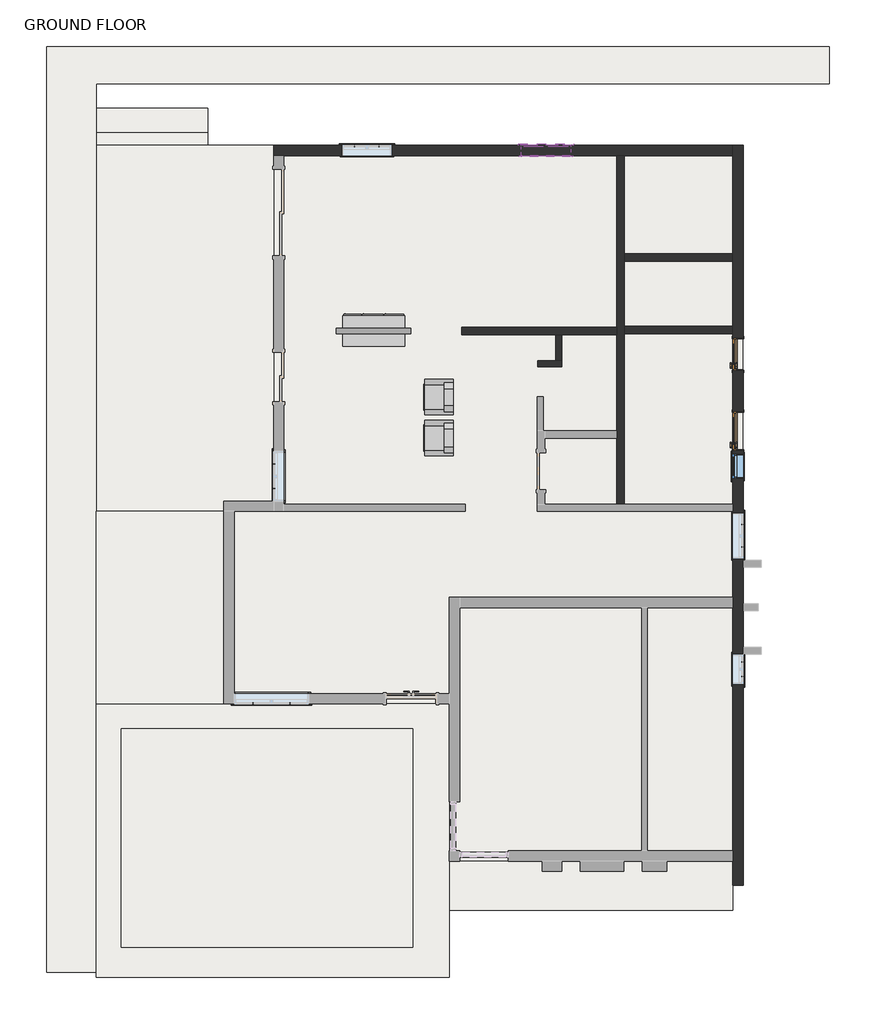
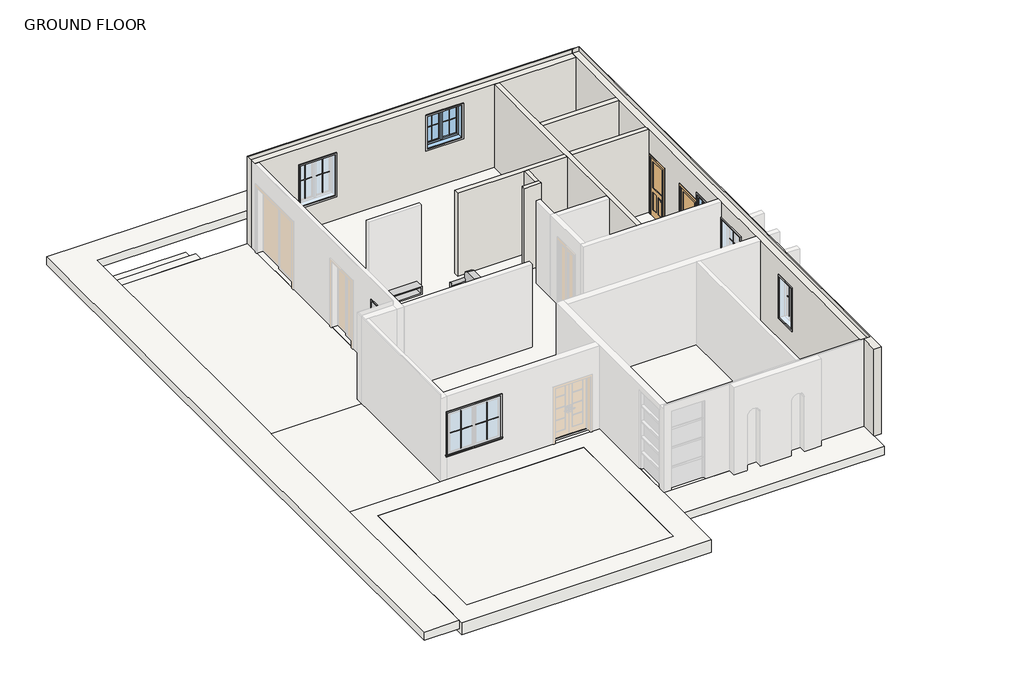
# One storey, part 2 of 2: 27 proxies, 9 slabs, 8 walls, 4 furniture elements, 2 doors, 2 windows.
"""IFC4 building model written with IfcOpenShell, lengths in millimetres."""

from ifc_helpers import new_model, si_unit, frame, origin, origin_with_axes, place, context, project, spatial, polyline, outline, extrude, faceted_brep, transform, mapped, element, save
from components import muntin_pattern_2x2_muntin_pattern_2x2_12159eb8, muntin_pattern_2x2_muntin_pattern_2x2_7b8f790b, muntin_pattern_2x2_muntin_pattern_2x2_a2bda2b8, muntin_pattern_2x2_muntin_pattern_2x2_5c299dc3, muntin_pattern_2x2_muntin_pattern_2x2_e751b040, muntin_pattern_2x2_muntin_pattern_2x2_9cc8fee8, muntin_pattern_2x2_muntin_pattern_2x2_4dfeb3f3, muntin_pattern_2x2_muntin_pattern_2x2_e852a7e4, muntin_pattern_2x2_muntin_pattern_2x2_8031e6f6, muntin_pattern_2x2_muntin_pattern_2x2_6dad3731, muntin_pattern_2x2_muntin_pattern_2x2_a30a3345, trim_window_exterior_flat_with_sill_dc35da0b, trim_window_exterior_flat_with_sill_683e4a0f, trim_window_exterior_flat_with_sill_c22f0c79, trim_window_exterior_flat_with_sill_7cfdd449, trim_window_exterior_flat_with_sill_4912eb0d, trim_window_exterior_flat_with_sill_92b9b949, trim_window_interior_flat_picture_frame_d06e6fc7, trim_window_interior_flat_picture_frame_4c1e0c81, trim_window_interior_flat_picture_frame_d1f4d6ef, trim_window_interior_flat_picture_frame_f1e0b15b, trim_window_interior_flat_picture_frame_978fd00d, trim_window_interior_flat_picture_frame_3bb882cf, door_2_5_90776985, door_3_192038f1, furniture_78335deb, chair_lounge_11461_couch_0866092f, family1_family1_08dda250, window_awning_single_2_9725ec62, window_casement_double_4_window_2_5590f608

model = new_model("IFC4")

# Units and contexts
model_context = context("Model", 3, world=origin())
ifc_project = project(units=[si_unit("LENGTHUNIT", "METRE", prefix="MILLI")], contexts=[model_context])

# Site, building, storey
site = spatial("IfcSite", under=ifc_project)
building = spatial("IfcBuilding", under=site)
storey = spatial("IfcBuildingStorey", under=building, Name="GROUND FLOOR", Elevation=457.2)

# Proxies
placement = place(None, origin())
muntin_pattern_2x2_muntin_pattern_2x2_shape = muntin_pattern_2x2_muntin_pattern_2x2_12159eb8(model_context)
element("IfcBuildingElementProxy", 1, Name="Muntin Pattern_2x2 : Muntin Pattern_2x2", ObjectType="Muntin Pattern_2x2 : Muntin Pattern_2x2", at=placement, inside=storey, context=model_context, shape_type="MappedRepresentation", body=[
    mapped(muntin_pattern_2x2_muntin_pattern_2x2_shape, transform((6234.5834916, 167.7933623, 1441.45), x_axis=(0.0, -1.0, 0.0), y_axis=(1.0, 0.0, 0.0), z_axis=(0.0, 0.0, 1.0))),
])
muntin_pattern_2x2_muntin_pattern_2x2_2_shape = muntin_pattern_2x2_muntin_pattern_2x2_7b8f790b(model_context)
element("IfcBuildingElementProxy", 2, Name="Muntin Pattern_2x2 : Muntin Pattern_2x2", ObjectType="Muntin Pattern_2x2 : Muntin Pattern_2x2", at=placement, inside=storey, context=model_context, shape_type="MappedRepresentation", body=[
    mapped(muntin_pattern_2x2_muntin_pattern_2x2_2_shape, transform((6234.5834916, -387.8316377, 1441.45), x_axis=(0.0, 1.0, 0.0), y_axis=(-1.0, 0.0, 0.0), z_axis=(0.0, 0.0, 1.0))),
])
muntin_pattern_2x2_muntin_pattern_2x2_3_shape = muntin_pattern_2x2_muntin_pattern_2x2_a2bda2b8(model_context)
element("IfcBuildingElementProxy", 3, Name="Muntin Pattern_2x2 : Muntin Pattern_2x2", ObjectType="Muntin Pattern_2x2 : Muntin Pattern_2x2", at=placement, inside=storey, context=model_context, shape_type="MappedRepresentation", body=[
    mapped(muntin_pattern_2x2_muntin_pattern_2x2_3_shape, transform((6234.5834916, -3204.4733398, 1441.45), x_axis=(0.0, -1.0, 0.0), y_axis=(1.0, 0.0, 0.0), z_axis=(0.0, 0.0, 1.0))),
])
muntin_pattern_2x2_muntin_pattern_2x2_4_shape = muntin_pattern_2x2_muntin_pattern_2x2_5c299dc3(model_context)
element("IfcBuildingElementProxy", 4, Name="Muntin Pattern_2x2 : Muntin Pattern_2x2", ObjectType="Muntin Pattern_2x2 : Muntin Pattern_2x2", at=placement, inside=storey, context=model_context, shape_type="MappedRepresentation", body=[
    mapped(muntin_pattern_2x2_muntin_pattern_2x2_4_shape, transform((6234.5834916, -3569.5983398, 1441.45), x_axis=(0.0, 1.0, 0.0), y_axis=(-1.0, 0.0, 0.0), z_axis=(0.0, 0.0, 1.0))),
])
muntin_pattern_2x2_muntin_pattern_2x2_5_shape = muntin_pattern_2x2_muntin_pattern_2x2_e751b040(model_context)
element("IfcBuildingElementProxy", 5, Name="Muntin Pattern_2x2 : Muntin Pattern_2x2", ObjectType="Muntin Pattern_2x2 : Muntin Pattern_2x2", at=placement, inside=storey, context=model_context, shape_type="MappedRepresentation", body=[
    mapped(muntin_pattern_2x2_muntin_pattern_2x2_5_shape, transform((-4883.0879467, -4227.6016767, 1441.45), x_axis=(-1.0, 0.0, 0.0), y_axis=(0.0, -1.0, 0.0), z_axis=(0.0, 0.0, 1.0))),
])
muntin_pattern_2x2_muntin_pattern_2x2_6_shape = muntin_pattern_2x2_muntin_pattern_2x2_9cc8fee8(model_context)
element("IfcBuildingElementProxy", 6, Name="Muntin Pattern_2x2 : Muntin Pattern_2x2", ObjectType="Muntin Pattern_2x2 : Muntin Pattern_2x2", at=placement, inside=storey, context=model_context, shape_type="MappedRepresentation", body=[
    mapped(muntin_pattern_2x2_muntin_pattern_2x2_6_shape, transform((-5794.3129467, -4227.6016767, 1441.45), x_axis=(1.0, 0.0, 0.0), y_axis=(0.0, 1.0, 0.0), z_axis=(0.0, 0.0, 1.0))),
])
muntin_pattern_2x2_muntin_pattern_2x2_7_shape = muntin_pattern_2x2_muntin_pattern_2x2_4dfeb3f3(model_context)
element("IfcBuildingElementProxy", 7, Name="Muntin Pattern_2x2 : Muntin Pattern_2x2", ObjectType="Muntin Pattern_2x2 : Muntin Pattern_2x2", at=placement, inside=storey, context=model_context, shape_type="MappedRepresentation", body=[
    mapped(muntin_pattern_2x2_muntin_pattern_2x2_7_shape, transform((1101.9313637, 9469.4685985, 2027.05), x_axis=(1.0, 0.0, 0.0), y_axis=(0.0, 1.0, 0.0), z_axis=(0.0, 0.0, 1.0))),
])
muntin_pattern_2x2_muntin_pattern_2x2_8_shape = muntin_pattern_2x2_muntin_pattern_2x2_e852a7e4(model_context)
element("IfcBuildingElementProxy", 8, Name="Muntin Pattern_2x2 : Muntin Pattern_2x2", ObjectType="Muntin Pattern_2x2 : Muntin Pattern_2x2", at=placement, inside=storey, context=model_context, shape_type="MappedRepresentation", body=[
    mapped(muntin_pattern_2x2_muntin_pattern_2x2_8_shape, transform((1708.3563637, 9469.4685985, 2027.05), x_axis=(-1.0, 0.0, 0.0), y_axis=(0.0, -1.0, 0.0), z_axis=(0.0, 0.0, 1.0))),
])
muntin_pattern_2x2_muntin_pattern_2x2_9_shape = muntin_pattern_2x2_muntin_pattern_2x2_8031e6f6(model_context)
element("IfcBuildingElementProxy", 9, Name="Muntin Pattern_2x2 : Muntin Pattern_2x2", ObjectType="Muntin Pattern_2x2 : Muntin Pattern_2x2", at=placement, inside=storey, context=model_context, shape_type="MappedRepresentation", body=[
    mapped(muntin_pattern_2x2_muntin_pattern_2x2_9_shape, transform((5999.6334916, 1597.0935985, 1441.45), x_axis=(0.0, 1.0, 0.0), y_axis=(-1.0, 0.0, 0.0), z_axis=(0.0, 0.0, 1.0))),
])
muntin_pattern_2x2_muntin_pattern_2x2_10_shape = muntin_pattern_2x2_muntin_pattern_2x2_6dad3731(model_context)
element("IfcBuildingElementProxy", 10, Name="Muntin Pattern_2x2 : Muntin Pattern_2x2", ObjectType="Muntin Pattern_2x2 : Muntin Pattern_2x2", at=placement, inside=storey, context=model_context, shape_type="MappedRepresentation", body=[
    mapped(muntin_pattern_2x2_muntin_pattern_2x2_10_shape, transform((-5278.2311363, 1047.5096373, 1441.45), x_axis=(0.0, 1.0, 0.0), y_axis=(-1.0, 0.0, 0.0), z_axis=(0.0, 0.0, 1.0))),
])
element("IfcBuildingElementProxy", 11, Name="Muntin Pattern_2x2 : Muntin Pattern_2x2", ObjectType="Muntin Pattern_2x2 : Muntin Pattern_2x2", at=placement, inside=storey, context=model_context, shape_type="MappedRepresentation", body=[
    mapped(muntin_pattern_2x2_muntin_pattern_2x2_10_shape, transform((-3299.7482334, 9469.4685985, 1441.45), x_axis=(1.0, 0.0, 0.0), y_axis=(0.0, 1.0, 0.0), z_axis=(0.0, 0.0, 1.0))),
])
muntin_pattern_2x2_muntin_pattern_2x2_11_shape = muntin_pattern_2x2_muntin_pattern_2x2_a30a3345(model_context)
element("IfcBuildingElementProxy", 12, Name="Muntin Pattern_2x2 : Muntin Pattern_2x2", ObjectType="Muntin Pattern_2x2 : Muntin Pattern_2x2", at=placement, inside=storey, context=model_context, shape_type="MappedRepresentation", body=[
    mapped(muntin_pattern_2x2_muntin_pattern_2x2_11_shape, transform((-5278.2311363, 1653.9346373, 1441.45), x_axis=(0.0, -1.0, 0.0), y_axis=(1.0, 0.0, 0.0), z_axis=(0.0, 0.0, 1.0))),
])
element("IfcBuildingElementProxy", 13, Name="Muntin Pattern_2x2 : Muntin Pattern_2x2", ObjectType="Muntin Pattern_2x2 : Muntin Pattern_2x2", at=placement, inside=storey, context=model_context, shape_type="MappedRepresentation", body=[
    mapped(muntin_pattern_2x2_muntin_pattern_2x2_11_shape, transform((-2693.3232334, 9469.4685985, 1441.45), x_axis=(-1.0, 0.0, 0.0), y_axis=(0.0, -1.0, 0.0), z_axis=(0.0, 0.0, 1.0))),
])
trim_window_exterior_flat_with_sill_shape = trim_window_exterior_flat_with_sill_dc35da0b(model_context)
element("IfcBuildingElementProxy", 14, Name="Trim-Window-Exterior-Flat : with Sill", ObjectType="Trim-Window-Exterior-Flat : with Sill", at=placement, inside=storey, context=model_context, shape_type="MappedRepresentation", body=[
    mapped(trim_window_exterior_flat_with_sill_shape, transform((6244.1084916, -110.0191377, 2895.6), x_axis=(0.0, 1.0, 0.0), y_axis=(0.0, 0.0, 1.0), z_axis=(1.0, 0.0, 0.0))),
])
trim_window_exterior_flat_with_sill_2_shape = trim_window_exterior_flat_with_sill_683e4a0f(model_context)
element("IfcBuildingElementProxy", 15, Name="Trim-Window-Exterior-Flat : with Sill", ObjectType="Trim-Window-Exterior-Flat : with Sill", at=placement, inside=storey, context=model_context, shape_type="MappedRepresentation", body=[
    mapped(trim_window_exterior_flat_with_sill_2_shape, transform((6244.1084916, -3387.0358398, 2895.6), x_axis=(0.0, 1.0, 0.0), y_axis=(0.0, 0.0, 1.0), z_axis=(1.0, 0.0, 0.0))),
])
trim_window_exterior_flat_with_sill_3_shape = trim_window_exterior_flat_with_sill_c22f0c79(model_context)
element("IfcBuildingElementProxy", 16, Name="Trim-Window-Exterior-Flat : with Sill", ObjectType="Trim-Window-Exterior-Flat : with Sill", at=placement, inside=storey, context=model_context, shape_type="MappedRepresentation", body=[
    mapped(trim_window_exterior_flat_with_sill_3_shape, transform((-5338.7004467, -4237.1266767, 2895.6), x_axis=(1.0, 0.0, 0.0), y_axis=(0.0, 0.0, 1.0), z_axis=(0.0, -1.0, 0.0))),
])
trim_window_exterior_flat_with_sill_4_shape = trim_window_exterior_flat_with_sill_7cfdd449(model_context)
element("IfcBuildingElementProxy", 17, Name="Trim-Window-Exterior-Flat : with Sill", ObjectType="Trim-Window-Exterior-Flat : with Sill", at=placement, inside=storey, context=model_context, shape_type="MappedRepresentation", body=[
    mapped(trim_window_exterior_flat_with_sill_4_shape, transform((1405.1438637, 9478.9935985, 3176.4), x_axis=(-1.0, 0.0, 0.0), y_axis=(0.0, 0.0, 1.0), z_axis=(0.0, 1.0, 0.0))),
])
trim_window_exterior_flat_with_sill_5_shape = trim_window_exterior_flat_with_sill_4912eb0d(model_context)
element("IfcBuildingElementProxy", 18, Name="Trim-Window-Exterior-Flat : with Sill", ObjectType="Trim-Window-Exterior-Flat : with Sill", at=placement, inside=storey, context=model_context, shape_type="MappedRepresentation", body=[
    mapped(trim_window_exterior_flat_with_sill_5_shape, transform((5990.1084916, 1597.0935985, 2895.6), x_axis=(0.0, -1.0, 0.0), y_axis=(0.0, 0.0, 1.0), z_axis=(-1.0, 0.0, 0.0))),
])
trim_window_exterior_flat_with_sill_6_shape = trim_window_exterior_flat_with_sill_92b9b949(model_context)
element("IfcBuildingElementProxy", 19, Name="Trim-Window-Exterior-Flat : with Sill", ObjectType="Trim-Window-Exterior-Flat : with Sill", at=placement, inside=storey, context=model_context, shape_type="MappedRepresentation", body=[
    mapped(trim_window_exterior_flat_with_sill_6_shape, transform((-5287.7561363, 1350.7221373, 2895.6), x_axis=(0.0, -1.0, 0.0), y_axis=(0.0, 0.0, 1.0), z_axis=(-1.0, 0.0, 0.0))),
])
element("IfcBuildingElementProxy", 20, Name="Trim-Window-Exterior-Flat : with Sill", ObjectType="Trim-Window-Exterior-Flat : with Sill", at=placement, inside=storey, context=model_context, shape_type="MappedRepresentation", body=[
    mapped(trim_window_exterior_flat_with_sill_6_shape, transform((-2996.5357334, 9478.9935985, 2895.6), x_axis=(-1.0, 0.0, 0.0), y_axis=(0.0, 0.0, 1.0), z_axis=(0.0, 1.0, 0.0))),
])
trim_window_interior_flat_picture_frame_shape = trim_window_interior_flat_picture_frame_d06e6fc7(model_context)
element("IfcBuildingElementProxy", 21, Name="Trim-Window-Interior-Flat : Picture Frame", ObjectType="Trim-Window-Interior-Flat : Picture Frame", at=placement, inside=storey, context=model_context, shape_type="MappedRepresentation", body=[
    mapped(trim_window_interior_flat_picture_frame_shape, transform((5990.1084916, -110.0191377, 2895.6), x_axis=(0.0, -1.0, 0.0), y_axis=(0.0, 0.0, 1.0), z_axis=(-1.0, 0.0, 0.0))),
])
trim_window_interior_flat_picture_frame_2_shape = trim_window_interior_flat_picture_frame_4c1e0c81(model_context)
element("IfcBuildingElementProxy", 22, Name="Trim-Window-Interior-Flat : Picture Frame", ObjectType="Trim-Window-Interior-Flat : Picture Frame", at=placement, inside=storey, context=model_context, shape_type="MappedRepresentation", body=[
    mapped(trim_window_interior_flat_picture_frame_2_shape, transform((5990.1084916, -3387.0358398, 2895.6), x_axis=(0.0, -1.0, 0.0), y_axis=(0.0, 0.0, 1.0), z_axis=(-1.0, 0.0, 0.0))),
])
trim_window_interior_flat_picture_frame_3_shape = trim_window_interior_flat_picture_frame_d1f4d6ef(model_context)
element("IfcBuildingElementProxy", 23, Name="Trim-Window-Interior-Flat : Picture Frame", ObjectType="Trim-Window-Interior-Flat : Picture Frame", at=placement, inside=storey, context=model_context, shape_type="MappedRepresentation", body=[
    mapped(trim_window_interior_flat_picture_frame_3_shape, transform((-5338.7004467, -3983.1266767, 2895.6), x_axis=(-1.0, 0.0, 0.0), y_axis=(0.0, 0.0, 1.0), z_axis=(0.0, 1.0, 0.0))),
])
trim_window_interior_flat_picture_frame_4_shape = trim_window_interior_flat_picture_frame_f1e0b15b(model_context)
element("IfcBuildingElementProxy", 24, Name="Trim-Window-Interior-Flat : Picture Frame", ObjectType="Trim-Window-Interior-Flat : Picture Frame", at=placement, inside=storey, context=model_context, shape_type="MappedRepresentation", body=[
    mapped(trim_window_interior_flat_picture_frame_4_shape, transform((1405.1438637, 9224.9935985, 3176.4), x_axis=(1.0, 0.0, 0.0), y_axis=(0.0, 0.0, 1.0), z_axis=(0.0, -1.0, 0.0))),
])
trim_window_interior_flat_picture_frame_5_shape = trim_window_interior_flat_picture_frame_978fd00d(model_context)
element("IfcBuildingElementProxy", 25, Name="Trim-Window-Interior-Flat : Picture Frame", ObjectType="Trim-Window-Interior-Flat : Picture Frame", at=placement, inside=storey, context=model_context, shape_type="MappedRepresentation", body=[
    mapped(trim_window_interior_flat_picture_frame_5_shape, transform((6244.1084916, 1597.0935985, 2895.6), x_axis=(0.0, 1.0, 0.0), y_axis=(0.0, 0.0, 1.0), z_axis=(1.0, 0.0, 0.0))),
])
trim_window_interior_flat_picture_frame_6_shape = trim_window_interior_flat_picture_frame_3bb882cf(model_context)
element("IfcBuildingElementProxy", 26, Name="Trim-Window-Interior-Flat : Picture Frame", ObjectType="Trim-Window-Interior-Flat : Picture Frame", at=placement, inside=storey, context=model_context, shape_type="MappedRepresentation", body=[
    mapped(trim_window_interior_flat_picture_frame_6_shape, transform((-5033.7561363, 1350.7221373, 2895.6), x_axis=(0.0, 1.0, 0.0), y_axis=(0.0, 0.0, 1.0), z_axis=(1.0, 0.0, 0.0))),
])
element("IfcBuildingElementProxy", 27, Name="Trim-Window-Interior-Flat : Picture Frame", ObjectType="Trim-Window-Interior-Flat : Picture Frame", at=placement, inside=storey, context=model_context, shape_type="MappedRepresentation", body=[
    mapped(trim_window_interior_flat_picture_frame_6_shape, transform((-2996.5357334, 9224.9935985, 2895.6), x_axis=(1.0, 0.0, 0.0), y_axis=(0.0, 0.0, 1.0), z_axis=(0.0, -1.0, 0.0))),
])

# Doors
door_2_5_shape = door_2_5_90776985(model_context)
element("IfcDoor", 28, ObjectType="2.5'", at=placement, inside=storey, context=model_context, shape_type="MappedRepresentation", body=[
    mapped(door_2_5_shape, transform((6113.9334916, 4345.0935985, 457.2), x_axis=(0.0, -1.0, 0.0), y_axis=(1.0, 0.0, 0.0), z_axis=(0.0, 0.0, 1.0))),
])
door_3_shape = door_3_192038f1(model_context)
element("IfcDoor", 29, ObjectType="3'", at=placement, inside=storey, context=model_context, shape_type="MappedRepresentation", body=[
    mapped(door_3_shape, transform((6113.9334916, 2460.6935985, 457.2), x_axis=(0.0, -1.0, 0.0), y_axis=(1.0, 0.0, 0.0), z_axis=(0.0, 0.0, 1.0))),
])

# Furniture
furniture_shape = furniture_78335deb(model_context)
element("IfcFurniture", 30, at=placement, inside=storey, context=model_context, shape_type="MappedRepresentation", body=[
    mapped(furniture_shape, transform((-2829.2809093, 5141.7322749, 457.2), x_axis=(-1.0, 0.0, 0.0), y_axis=(0.0, -1.0, 0.0), z_axis=(0.0, 0.0, 1.0))),
])
chair_lounge_11461_couch_shape = chair_lounge_11461_couch_0866092f(model_context)
element("IfcFurniture", 31, ObjectType="Chair-Lounge_11461 : Couch", at=placement, inside=storey, context=model_context, shape_type="MappedRepresentation", body=[
    mapped(chair_lounge_11461_couch_shape, transform((-874.5061363, 2290.7935985, 457.2), x_axis=(0.0, -1.0, 0.0), y_axis=(1.0, 0.0, 0.0), z_axis=(0.0, 0.0, 1.0))),
])
element("IfcFurniture", 32, ObjectType="Chair-Lounge_11461 : Couch", at=placement, inside=storey, context=model_context, shape_type="MappedRepresentation", body=[
    mapped(chair_lounge_11461_couch_shape, transform((-874.5061363, 3294.0935985, 457.2), x_axis=(0.0, -1.0, 0.0), y_axis=(1.0, 0.0, 0.0), z_axis=(0.0, 0.0, 1.0))),
])
family1_family1_shape = family1_family1_08dda250(model_context)
element("IfcFurniture", 33, ObjectType="Family1 : Family1", at=placement, inside=storey, context=model_context, shape_type="MappedRepresentation", body=[
    mapped(family1_family1_shape, transform((-2829.2809093, 4849.6322749, 457.2), x_axis=(-1.0, 0.0, 0.0), y_axis=(0.0, -1.0, 0.0), z_axis=(0.0, 0.0, 1.0))),
])

# Slabs
element("IfcSlab", 34, ObjectType="6\"", at=placement, inside=storey, context=model_context, shape_type="SweptSolid", body=[
    extrude(outline(polyline([(-5287.7561363, 9478.9935985), (-5287.7561363, 741.1221373), (-6507.1004467, 741.1221373), (-6507.1004467, 487.1221375), (-9643.8561363, 487.1221375), (-9643.8561363, 9478.9935985), (-5287.7561363, 9478.9935985)])), origin_with_axes(), (0.0, 0.0, 1.0), 457.2),
])
element("IfcSlab", 35, ObjectType="6\" 3", at=placement, inside=storey, context=model_context, shape_type="SweptSolid", body=[
    extrude(outline(polyline([(-6900.6561363, 9478.9935985), (-9643.8561363, 9478.9935985), (-9643.8561363, 10393.3935985), (-6900.6561363, 10393.3935985), (-6900.6561363, 9478.9935985)])), origin_with_axes(), (0.0, 0.0, 1.0), 152.4),
])
element("IfcSlab", 36, ObjectType="6\" 3", at=placement, inside=storey, context=model_context, shape_type="SweptSolid", body=[
    extrude(outline(polyline([(-6900.6561363, 9478.9935985), (-9643.8561363, 9478.9935985), (-9643.8561363, 9783.7935985), (-6900.6561363, 9783.7935985), (-6900.6561363, 9478.9935985)])), frame((0.0, 0.0, 304.8), z_axis=(0.0, 0.0, 1.0), x_axis=(1.0, 0.0, 0.0)), (0.0, 0.0, 1.0), 152.4),
])
element("IfcSlab", 37, ObjectType="6\" 4", at=placement, inside=storey, context=model_context, shape_type="SweptSolid", body=[
    extrude(outline(polyline([(-6507.1004467, 487.1221375), (-6507.1004467, -4237.1266767), (-9643.8561363, -4237.1266767), (-9643.8561363, 487.1221375), (-6507.1004467, 487.1221375)])), origin_with_axes(), (0.0, 0.0, 1.0), 457.2),
])
element("IfcSlab", 38, ObjectType="6\" 5", at=placement, inside=storey, context=model_context, shape_type="SweptSolid", body=[
    extrude(outline(polyline([(-1864.8415084, -4846.7266767), (-1864.8415084, -10218.7064015), (-9034.2561363, -10218.7064015), (-9034.2561363, -4846.7266767), (-1864.8415084, -4846.7266767)])), origin_with_axes(), (0.0, 0.0, 1.0), 457.2),
])
element("IfcSlab", 39, ObjectType="6\" 6", at=placement, inside=storey, context=model_context, shape_type="SweptSolid", body=[
    extrude(outline(polyline([(-969.7561363, -4237.1266767), (-969.7561363, -10955.3064015), (-9643.8561363, -10955.3064015), (-9643.8561363, -4237.1266767), (-969.7561363, -4237.1266767)]), holes=[polyline([(-1864.8415084, -4846.7266767), (-9034.2561363, -4846.7266767), (-9034.2561363, -10218.7064015), (-1864.8415084, -10218.7064015), (-1864.8415084, -4846.7266767)])]), origin_with_axes(), (0.0, 0.0, 1.0), 457.2),
])
element("IfcSlab", 40, ObjectType="GRASS", at=placement, inside=storey, context=model_context, shape_type="SweptSolid", body=[
    extrude(outline(polyline([(-10863.0561363, -10828.3064015), (-10863.0561363, 11904.6935985), (-9643.8561363, 11904.6935985), (8352.5731195, 11904.6935985), (8352.5731195, 10990.2935985), (-9643.8561363, 10990.2935985), (-9643.8561363, -10828.3064015), (-10863.0561363, -10828.3064015)])), frame((0.0, 0.0, 152.4), z_axis=(0.0, 0.0, 1.0), x_axis=(1.0, 0.0, 0.0)), (0.0, 0.0, 1.0), 304.8),
])
element("IfcSlab", 41, ObjectType="GRASS", at=placement, inside=storey, context=model_context, shape_type="SweptSolid", body=[
    extrude(outline(polyline([(5990.1084916, -9304.3064015), (-969.7561363, -9304.3064015), (-969.7561363, -8097.8064015), (5990.1084916, -8097.8064015), (5990.1084916, -9304.3064015)])), frame((0.0, 0.0, 152.4), z_axis=(0.0, 0.0, 1.0), x_axis=(1.0, 0.0, 0.0)), (0.0, 0.0, 1.0), 304.8),
])
element("IfcSlab", 42, ObjectType="INTERIOR TILES", at=placement, inside=storey, context=model_context, shape_type="Brep", body=[
    faceted_brep([(-5275.0561363, 9466.0221373, 0.0), (6231.1438637, 9466.0221373, 0.0), (6231.1438637, -8085.3778627, 0.0), (5990.1084916, -8085.3778627, 0.0), (-715.7561363, -8085.3778627, 0.0), (-957.0561363, -8085.3778627, 0.0), (-957.0561363, -4224.5778627, 0.0), (-969.7561363, -4224.5778627, 0.0), (-6253.1004467, -4224.5778627, 0.0), (-6494.2561363, -4224.5778627, 0.0), (-6494.2561363, 487.1221373, 0.0), (-6494.2561363, 728.4221373, 0.0), (-5287.7561363, 728.4221373, 0.0), (-5275.0561363, 728.4221373, 0.0), (-5275.0561363, 9224.9935985, 0.0), (-5275.0561363, 9466.0221373, 457.2), (-5275.0561363, 9224.9935985, 457.2), (-5275.0561363, 728.4221373, 457.2), (-5287.7561363, 728.4221373, 457.2), (-6494.2561363, 728.4221373, 457.2), (-6494.2561363, 487.1221373, 457.2), (-6494.2561363, -4224.5778627, 457.2), (-6253.1004467, -4224.5778627, 457.2), (-969.7561363, -4224.5778627, 457.2), (-957.0561363, -4224.5778627, 457.2), (-957.0561363, -8085.3778627, 457.2), (-715.7561363, -8085.3778627, 457.2), (5990.1084916, -8085.3778627, 457.2), (6231.1438637, -8085.3778627, 457.2), (6231.1438637, 9466.0221373, 457.2)], [[[0, 1, 2, 3, 4, 5, 6, 7, 8, 9, 10, 11, 12, 13, 14]], [[15, 16, 17, 18, 19, 20, 21, 22, 23, 24, 25, 26, 27, 28, 29]], [[1, 0, 15, 29]], [[2, 1, 29, 28]], [[5, 4, 3, 2, 28, 27, 26, 25]], [[6, 5, 25, 24]], [[9, 8, 7, 6, 24, 23, 22, 21]], [[11, 10, 9, 21, 20, 19]], [[13, 12, 11, 19, 18, 17]], [[0, 14, 13, 17, 16, 15]]]),
])

# Walls
element("IfcWall", 43, ObjectType="4.5\"", at=placement, inside=storey, context=model_context, shape_type="Brep", body=[
    faceted_brep([(1201.9438637, 4042.9709514, 457.2), (1786.1438637, 4042.9709514, 457.2), (1786.1438637, 4042.9709514, 3505.2), (1201.9438637, 4042.9709514, 3505.2), (1786.1438637, 4182.6709514, 457.2), (1646.4438637, 4182.6709514, 457.2), (1201.9438637, 4182.6709514, 457.2), (1201.9438637, 4182.6709514, 3505.2), (1786.1438637, 4182.6709514, 3505.2)], [[[0, 1, 2, 3]], [[4, 5, 6, 7, 8]], [[1, 0, 6, 5, 4]], [[6, 0, 3, 7]], [[1, 4, 8, 2]], [[3, 2, 8, 7]]]),
])
element("IfcWall", 44, ObjectType="4.5\"", at=placement, inside=storey, context=model_context, shape_type="SweptSolid", body=[
    extrude(outline(polyline([(1786.1438637, 4830.5822749), (1786.1438637, 4182.6709514), (1646.4438637, 4182.6709514), (1646.4438637, 4830.5822749), (1786.1438637, 4830.5822749)])), frame((0.0, 0.0, 457.2), z_axis=(0.0, 0.0, 1.0), x_axis=(1.0, 0.0, 0.0)), (0.0, 0.0, 1.0), 3048.0),
])
element("IfcWall", 45, ObjectType="6\" WALL", at=placement, inside=storey, context=model_context, shape_type="Brep", body=[
    faceted_brep([(3322.8438637, 665.1935985, 457.2), (3322.8438637, 4856.1935985, 457.2), (3322.8438637, 5033.9935985, 457.2), (3322.8438637, 6634.1935985, 457.2), (3322.8438637, 6811.9935985, 457.2), (3322.8438637, 9224.9935985, 457.2), (3322.8438637, 9224.9935985, 3505.2), (3322.8438637, 665.1935985, 3505.2), (3145.0438637, 9224.9935985, 457.2), (3145.0438637, 5008.3822749, 457.2), (3145.0438637, 4830.5822749, 457.2), (3145.0438637, 2468.5935985, 457.2), (3145.0438637, 2290.7935985, 457.2), (3145.0438637, 665.1935985, 457.2), (3145.0438637, 665.1935985, 3505.2), (3145.0438637, 2290.7935985, 3505.2), (3145.0438637, 2468.5935985, 3505.2), (3145.0438637, 4830.5822749, 3505.2), (3145.0438637, 5008.3822749, 3505.2), (3145.0438637, 9224.9935985, 3505.2)], [[[0, 1, 2, 3, 4, 5, 6, 7]], [[8, 9, 10, 11, 12, 13, 14, 15, 16, 17, 18, 19]], [[5, 4, 3, 2, 1, 0, 13, 12, 11, 10, 9, 8]], [[5, 8, 19, 6]], [[13, 0, 7, 14]], [[7, 6, 19, 18, 17, 16, 15, 14]]]),
])
element("IfcWall", 46, ObjectType="6\" WALL", at=placement, inside=storey, context=model_context, shape_type="SweptSolid", body=[
    extrude(outline(polyline([(5990.1084916, 6634.1935985), (3322.8438637, 6634.1935985), (3322.8438637, 6811.9935985), (5990.1084916, 6811.9935985), (5990.1084916, 6634.1935985)])), frame((0.0, 0.0, 457.2), z_axis=(0.0, 0.0, 1.0), x_axis=(1.0, 0.0, 0.0)), (0.0, 0.0, 1.0), 3048.0),
])
element("IfcWall", 47, ObjectType="6\" WALL", at=placement, inside=storey, context=model_context, shape_type="SweptSolid", body=[
    extrude(outline(polyline([(5990.1084916, 4856.1935985), (3322.8438637, 4856.1935985), (3322.8438637, 5033.9935985), (5990.1084916, 5033.9935985), (5990.1084916, 4856.1935985)])), frame((0.0, 0.0, 457.2), z_axis=(0.0, 0.0, 1.0), x_axis=(1.0, 0.0, 0.0)), (0.0, 0.0, 1.0), 3048.0),
])
element("IfcWall", 48, ObjectType="6\" WALL", at=placement, inside=storey, context=model_context, shape_type="Brep", body=[
    faceted_brep([(3145.0438637, 5008.3822749, 457.2), (-664.9561363, 5008.3822749, 457.2), (-664.9561363, 5008.3822749, 3505.2), (3145.0438637, 5008.3822749, 3505.2), (-664.9561363, 4830.5822749, 457.2), (1646.4438637, 4830.5822749, 457.2), (1786.1438637, 4830.5822749, 457.2), (3145.0438637, 4830.5822749, 457.2), (3145.0438637, 4830.5822749, 3505.2), (1786.1438637, 4830.5822749, 3505.2), (1646.4438637, 4830.5822749, 3505.2), (-664.9561363, 4830.5822749, 3505.2)], [[[0, 1, 2, 3]], [[4, 5, 6, 7, 8, 9, 10, 11]], [[1, 0, 7, 6, 5, 4]], [[1, 4, 11, 2]], [[7, 0, 3, 8]], [[3, 2, 11, 10, 9, 8]]]),
])
element("IfcWall", 49, ObjectType="9\"", at=placement, inside=storey, context=model_context, shape_type="Brep", body=[
    faceted_brep([(5990.1084916, -8694.7064015, 457.2), (5990.1084916, -8694.7064015, 3657.6), (5990.1084916, -8097.8064015, 3657.6), (5990.1084916, -8085.1064015, 3657.6), (5990.1084916, -8085.1064015, 3505.2), (5990.1084916, -1874.8064015, 3505.2), (5990.1084916, -1620.8064015, 3505.2), (5990.1084916, 487.3935985, 3505.2), (5990.1084916, 665.1935985, 3505.2), (5990.1084916, 4856.1935985, 3505.2), (5990.1084916, 5033.9935985, 3505.2), (5990.1084916, 6634.1935985, 3505.2), (5990.1084916, 6811.9935985, 3505.2), (5990.1084916, 9466.2935985, 3505.2), (5990.1084916, 9466.2935985, 3657.6), (5990.1084916, 9478.9935985, 3657.6), (5990.1084916, 9478.9935985, 457.2), (5990.1084916, 9224.9935985, 457.2), (5990.1084916, 6811.9935985, 457.2), (5990.1084916, 6634.1935985, 457.2), (5990.1084916, 5033.9935985, 457.2), (5990.1084916, 4856.1935985, 457.2), (5990.1084916, 4751.4935985, 457.2), (5990.1084916, 4751.4935985, 2616.2), (5990.1084916, 3938.6935985, 2616.2), (5990.1084916, 3938.6935985, 457.2), (5990.1084916, 2943.2935985, 457.2), (5990.1084916, 2943.2935985, 2616.2), (5990.1084916, 1978.0935985, 2616.2), (5990.1084916, 1978.0935985, 457.2), (5990.1084916, 665.1935985, 457.2), (5990.1084916, 487.3935985, 457.2), (5990.1084916, -1620.8064015, 457.2), (5990.1084916, -1874.8064015, 457.2), (5990.1084916, -7843.8064015, 457.2), (5990.1084916, -8097.8064015, 457.2), (5990.1084916, -668.8191377, 2895.6), (5990.1084916, -668.8191377, 1371.6), (5990.1084916, 448.7808623, 1371.6), (5990.1084916, 448.7808623, 2895.6), (5990.1084916, -3755.3358398, 2895.6), (5990.1084916, -3755.3358398, 1371.6), (5990.1084916, -3018.7358398, 1371.6), (5990.1084916, -3018.7358398, 2895.6), (5990.1084916, 1901.8935985, 1371.6), (5990.1084916, 1901.8935985, 2895.6), (5990.1084916, 1292.2935985, 2895.6), (5990.1084916, 1292.2935985, 1371.6), (6244.1084916, -8694.7064015, 3657.6), (6244.1084916, -8694.7064015, 457.2), (6244.1084916, -3018.7358398, 457.2), (6244.1084916, -2840.9358398, 457.2), (6244.1084916, -1952.0318739, 457.2), (6244.1084916, -1774.2318739, 457.2), (6244.1084916, -885.2318739, 457.2), (6244.1084916, -707.4318739, 457.2), (6244.1084916, 1978.0935985, 457.2), (6244.1084916, 1978.0935985, 2616.2), (6244.1084916, 2943.2935985, 2616.2), (6244.1084916, 2943.2935985, 457.2), (6244.1084916, 3938.6935985, 457.2), (6244.1084916, 3938.6935985, 2616.2), (6244.1084916, 4751.4935985, 2616.2), (6244.1084916, 4751.4935985, 457.2), (6244.1084916, 9478.9935985, 457.2), (6244.1084916, 9478.9935985, 3657.6), (6244.1084916, -707.4318739, 3657.6), (6244.1084916, -885.2318739, 3657.6), (6244.1084916, -1774.2318739, 3657.6), (6244.1084916, -1952.0318739, 3657.6), (6244.1084916, -2840.9358398, 3657.6), (6244.1084916, -3018.7358398, 3657.6), (6244.1084916, -668.8191377, 1371.6), (6244.1084916, -668.8191377, 2895.6), (6244.1084916, 448.7808623, 2895.6), (6244.1084916, 448.7808623, 1371.6), (6244.1084916, -3755.3358398, 1371.6), (6244.1084916, -3755.3358398, 2895.6), (6244.1084916, -3018.7358398, 2895.6), (6244.1084916, -3018.7358398, 1371.6), (6244.1084916, 1901.8935985, 2895.6), (6244.1084916, 1901.8935985, 1371.6), (6244.1084916, 1292.2935985, 1371.6), (6244.1084916, 1292.2935985, 2895.6), (6218.7084916, 9466.2935985, 3657.6), (6218.7084916, -8085.1064015, 3657.6), (6218.7084916, -8085.1064015, 3505.2), (6218.7084916, 9466.2935985, 3505.2)], [[[0, 1, 2, 3, 4, 5, 6, 7, 8, 9, 10, 11, 12, 13, 14, 15, 16, 17, 18, 19, 20, 21, 22, 23, 24, 25, 26, 27, 28, 29, 30, 31, 32, 33, 34, 35], [36, 37, 38, 39], [40, 41, 42, 43], [44, 45, 46, 47]], [[48, 49, 50, 51, 52, 53, 54, 55, 56, 57, 58, 59, 60, 61, 62, 63, 64, 65, 66, 67, 68, 69, 70, 71], [72, 73, 74, 75], [76, 77, 78, 79], [80, 81, 82, 83]], [[16, 64, 63, 22, 21, 20, 19, 18, 17]], [[49, 0, 35, 34, 33, 32, 31, 30, 29, 56, 55, 54, 53, 52, 51, 50]], [[25, 60, 59, 26]], [[1, 0, 49, 48]], [[48, 71, 70, 69, 68, 67, 66, 65, 15, 14, 84, 85, 3, 2, 1]], [[16, 15, 65, 64]], [[37, 36, 73, 72]], [[38, 37, 72, 75]], [[39, 38, 75, 74]], [[36, 39, 74, 73]], [[41, 40, 77, 76]], [[42, 41, 76, 79]], [[43, 42, 79, 78]], [[40, 43, 78, 77]], [[24, 61, 60, 25]], [[61, 24, 23, 62]], [[62, 23, 22, 63]], [[28, 57, 56, 29]], [[57, 28, 27, 58]], [[58, 27, 26, 59]], [[81, 80, 45, 44]], [[82, 81, 44, 47]], [[83, 82, 47, 46]], [[80, 83, 46, 45]], [[86, 87, 13, 12, 11, 10, 9, 8, 7, 6, 5, 4]], [[87, 86, 85, 84]], [[85, 86, 4, 3]], [[87, 84, 14, 13]]]),
])
element("IfcWall", 50, ObjectType="9\"", at=placement, inside=storey, context=model_context, shape_type="Brep", body=[
    faceted_brep([(5990.1084916, 9478.9935985, 457.2), (-5287.7561363, 9478.9935985, 457.2), (-5287.7561363, 9478.9935985, 3657.6), (5990.1084916, 9478.9935985, 3657.6), (-2386.9357334, 9478.9935985, 1371.6), (-2386.9357334, 9478.9935985, 2895.6), (-3606.1357334, 9478.9935985, 2895.6), (-3606.1357334, 9478.9935985, 1371.6), (2014.7438637, 9478.9935985, 1957.2), (2014.7438637, 9478.9935985, 3176.4), (795.5438637, 9478.9935985, 3176.4), (795.5438637, 9478.9935985, 1957.2), (-5287.7561363, 9224.9935985, 457.2), (-5033.7561363, 9224.9935985, 457.2), (3145.0438637, 9224.9935985, 457.2), (3322.8438637, 9224.9935985, 457.2), (5990.1084916, 9224.9935985, 457.2), (5990.1084916, 9224.9935985, 3505.2), (3322.8438637, 9224.9935985, 3505.2), (3145.0438637, 9224.9935985, 3505.2), (-5033.7561363, 9224.9935985, 3505.2), (-5275.0561363, 9224.9935985, 3505.2), (-5275.0561363, 9224.9935985, 3657.6), (-5287.7561363, 9224.9935985, 3657.6), (-2386.9357334, 9224.9935985, 2895.6), (-2386.9357334, 9224.9935985, 1371.6), (-3606.1357334, 9224.9935985, 1371.6), (-3606.1357334, 9224.9935985, 2895.6), (2014.7438637, 9224.9935985, 3176.4), (2014.7438637, 9224.9935985, 1957.2), (795.5438637, 9224.9935985, 1957.2), (795.5438637, 9224.9935985, 3176.4), (-5275.0561363, 9466.2935985, 3657.6), (5990.1084916, 9466.2935985, 3657.6), (5990.1084916, 9466.2935985, 3505.2), (-5275.0561363, 9466.2935985, 3505.2)], [[[0, 1, 2, 3], [4, 5, 6, 7], [8, 9, 10, 11]], [[12, 13, 14, 15, 16, 17, 18, 19, 20, 21, 22, 23], [24, 25, 26, 27], [28, 29, 30, 31]], [[1, 0, 16, 15, 14, 13, 12]], [[3, 2, 23, 22, 32, 33]], [[0, 3, 33, 34, 17, 16]], [[2, 1, 12, 23]], [[25, 24, 5, 4]], [[26, 25, 4, 7]], [[27, 26, 7, 6]], [[24, 27, 6, 5]], [[8, 29, 28, 9]], [[29, 8, 11, 30]], [[30, 11, 10, 31]], [[9, 28, 31, 10]], [[34, 35, 21, 20, 19, 18, 17]], [[32, 35, 34, 33]], [[35, 32, 22, 21]]]),
])

# Windows
window_awning_single_2_shape = window_awning_single_2_9725ec62(model_context)
element("IfcWindow", 51, ObjectType="Window-Awning-Single : 2'", at=placement, inside=storey, context=model_context, shape_type="MappedRepresentation", body=[
    mapped(window_awning_single_2_shape, transform((6117.1084916, 1597.0935985, 457.2), x_axis=(0.0, 1.0, 0.0), y_axis=(-1.0, 0.0, 0.0), z_axis=(0.0, 0.0, 1.0))),
])
window_casement_double_4_window_2_shape = window_casement_double_4_window_2_5590f608(model_context)
element("IfcWindow", 52, ObjectType="Window-Casement-Double : 4 window 2", at=placement, inside=storey, context=model_context, shape_type="MappedRepresentation", body=[
    mapped(window_casement_double_4_window_2_shape, transform((1405.1438637, 9351.9935985, 1042.8), x_axis=(1.0, 0.0, 0.0), y_axis=(0.0, 1.0, 0.0), z_axis=(0.0, 0.0, 1.0))),
])

save(model, "model.ifc")

# Revit data of these elements
# Type "Muntin Pattern_2x2 : Muntin Pattern_2x2"
#   Width [instance default] = 4' - 0"
#   Thickness = 0' - 0 1/2"
#   Height [instance default] = 4' - 0"
#   Distance = 0' - 0 3/4"
#   Interior Material [instance default] = none
#   Exterior Material [instance default] = none
#   Default Elevation = 0
# Type "Trim-Window-Exterior-Flat : with Sill"
#   Trim Width = 0' - 2 1/4"
#   Trim Thickness_Picture Frame = 0' - 1 1/4"
#   Trim Thickness_with Sill = 0' - 0 3/4"
#   Sill Thickness = 0' - 1 1/4"
#   Opening Width [instance default] = 2' - 0"
#   Opening Height [instance default] = 3' - 0"
#   Default Elevation = 4' - 0"
#   Sill = yes
#   Picture Frame = no
#   Trim Material [instance default] = none
# Type "Trim-Window-Interior-Flat : Picture Frame"
#   Trim Thickness_Picture Frame = 0' - 1 1/4"
#   Trim Width = 0' - 2 1/4"
#   Trim Thickness_with Sill = 0' - 0 3/4"
#   Sill Thickness = 0' - 1 1/4"
#   Opening Width [instance default] = 2' - 0"
#   Opening Height [instance default] = 3' - 0"
#   Default Elevation = 4' - 0"
#   Sill = no
#   Picture Frame = yes
#   Trim Material [instance default] = none
# Type "2.5'"
#   Type Mark = "11"
#   Assembly Code = "B2030100"
#   Analytic Construction = "French door, wood frame with single glass"
#   Top Rail = 0' - 4 3/4"
#   Threshold Offset [instance default] = 0' - 0 1/2"
#   Thickness = 0' - 1 3/8"
#   Thermal Resistance (R) = 1.0696 (h·ft²·°F)/BTU
#   Swing Angle [instance default] = 90.00°
#   Stiles = 0' - 4 3/4"
#   Rough Width = 2' - 8"
#   Rough Height = 7' - 1"
#   Lock Rail = 0' - 7 1/8"
#   Height = 7' - 0"
#   Width = 2' - 6"
#   Heat Transfer Coefficient (U) = 0.9350 BTU/(h·ft²·°F)
#   Door Offset [instance default] = 0' - 0"
#   Bottom Rail = 0' - 9 1/2"
#   Threshold [instance default] = yes
#   Function = 1
#   Exterior Trim [instance default] = yes
#   Trim Material = Cherry
#   Threshold Material = Cherry
#   Panel Material = Cherry
#   Glazing = Glass
#   Frame Material = Cherry
#   Door Handle Material = Aluminum
#   Visual Light Transmittance = 0
#   Solar Heat Gain Coefficient = 0
#   Wall Closure = (empty or 0)
#   Construction Type = (empty or 0)
# Type "3'"
#   Type Mark = "12"
#   Assembly Code = "B2030100"
#   Analytic Construction = "French door, wood frame with single glass"
#   Top Rail = 0' - 4 3/4"
#   Threshold Offset [instance default] = 0' - 0 1/2"
#   Thickness = 0' - 1 3/8"
#   Thermal Resistance (R) = 1.0696 (h·ft²·°F)/BTU
#   Swing Angle [instance default] = 90.00°
#   Stiles = 0' - 4 3/4"
#   Rough Width = 3' - 2"
#   Rough Height = 7' - 1"
#   Lock Rail = 0' - 7 1/8"
#   Height = 7' - 0"
#   Width = 3' - 0"
#   Heat Transfer Coefficient (U) = 0.9350 BTU/(h·ft²·°F)
#   Door Offset [instance default] = 0' - 0"
#   Bottom Rail = 0' - 9 1/2"
#   Threshold [instance default] = yes
#   Function = 1
#   Exterior Trim [instance default] = yes
#   Trim Material = Cherry
#   Threshold Material = Cherry
#   Panel Material = Cherry
#   Glazing = Glass
#   Frame Material = Cherry
#   Door Handle Material = Aluminum
#   Visual Light Transmittance = 0
#   Solar Heat Gain Coefficient = 0
#   Wall Closure = (empty or 0)
#   Construction Type = (empty or 0)
# Type
#   Default Elevation = 0
# Type "Chair-Lounge_11461 : Couch"
#   Default Elevation = 0
#   Assembly Code = ""
# Type "Family1 : Family1"
#   Default Elevation = 0
# Type "6\""
#   Assembly Code = "B1010"
#   Function = 0
#   Layers, outside or top first: 1' - 6" "WOOD FLOOR" (function 1)
# Type "6\" 3"
#   Assembly Code = "B1010"
#   Function = 0
#   Layers, outside or top first: 0' - 6" "Concrete, Cast-in-Place gray" (function 1)
# Type "6\" 4"
#   Assembly Code = "B1010"
#   Function = 0
#   Layers, outside or top first: 1' - 6" "WALKING AREA TILES(1)" (function 1)
# Type "6\" 5"
#   Assembly Code = "B1010"
#   Function = 0
#   Layers, outside or top first: 1' - 6" "WALKING AREA TILES(1)" (function 1)
# Type "6\" 6"
#   Assembly Code = "B1010"
#   Function = 0
#   Layers, outside or top first: 1' - 6" "WALKING AREA TILES" (function 1)
# Type "GRASS"
#   Assembly Code = "B1010"
#   Function = 0
#   Layers, outside or top first: 1' - 0" "Grass" (function 1)
# Type "INTERIOR TILES"
#   Assembly Code = "B1010"
#   Function = 0
#   Layers, outside or top first: 1' - 6" "INTERIOR TILE" (function 1)
# Type "4.5\""
#   Assembly Code = "B2010"
#   Layers, outside or top first: 0' - 0 1/2" no material (function 4); 0' - 4 1/2" "Acoustic Ceiling Tile 24 x 24" (function 1); 0' - 0 1/2" no material (function 4)
# Type "6\" WALL"
#   Assembly Code = "B2010"
#   Layers, outside or top first: 0' - 0 1/2" no material (function 4); 0' - 6" no material (function 1); 0' - 0 1/2" no material (function 4)
# Type "9\""
#   Assembly Code = "B2010"
#   Layers, outside or top first: 0' - 0 1/2" no material (function 4); 0' - 9" no material (function 1); 0' - 0 1/2" no material (function 4)
# Type "Window-Awning-Single : 2'"
#   Type Mark = "24"
#   Fire Rating = "0.5h"
#   Assembly Code = "B2020100"
#   Analytic Construction = "Double glazing - domestic"
#   Window Inset [instance default] = 0' - 0"
#   Wall Thickness [instance default] = 0' - 6"
#   Visual Light Transmittance = 0.81
#   Thermal Resistance (R) = 1.8146 (h·ft²·°F)/BTU
#   Solar Heat Gain Coefficient = 0.76
#   Rough Width = 2' - 0 1/2"
#   Rough Height = 5' - 0 1/2"
#   Interior Wall Closure [instance default] = 0' - 2 1/4"
#   Height = 5' - 0"
#   Heat Transfer Coefficient (U) = 0.5511 BTU/(h·ft²·°F)
#   Frame Extension [instance default] = 0' - 0 1/4"
#   Exterior Wall Closure [instance default] = 0' - 1 1/4"
#   Extension Jamb [instance default] = 0' - 2 1/4"
#   Default Sill Height = 3' - 0"
#   Width = 2' - 0"
#   Muntin Visibility = yes
#   Interior Trim Visibility [instance default] = yes
#   Exterior Trim Visibility [instance default] = yes
#   Extension Jamb Visibility [instance default] = yes
#   Muntin Pattern = Muntin Pattern_2x2 : Muntin Pattern_2x2
#   Interior Trim Material = Wood - Stained
#   Interior Trim = Trim-Window-Interior-Flat : Picture Frame
#   Interior Frame Material = Wood - Stained
#   Glass Panel Material = Glass
#   Exterior Trim Material = Clad - White
#   Exterior Trim = Trim-Window-Exterior-Flat : with Sill
#   Exterior Frame Material = Clad - White
#   Wall Closure = (empty or 0)
# Type "Window-Casement-Double : 4 window 2"
#   Type Mark = "22"
#   Fire Rating = "0.5h"
#   Assembly Code = "B2020100"
#   Analytic Construction = "Double glazing - domestic"
#   Frame Extension [instance default] = 0' - 0 1/4"
#   Window Inset [instance default] = 0' - 0"
#   Wall Thickness [instance default] = 0' - 6"
#   Interior Wall Closure [instance default] = 0' - 2 1/4"
#   Half Width = 2' - 0"
#   Visual Light Transmittance = 0.81
#   Thermal Resistance (R) = 1.8146 (h·ft²·°F)/BTU
#   Solar Heat Gain Coefficient = 0.76
#   Rough Width = 4' - 0 1/2"
#   Rough Height = 4' - 0 1/2"
#   Height = 4' - 0"
#   Heat Transfer Coefficient (U) = 0.5511 BTU/(h·ft²·°F)
#   Exterior Wall Closure [instance default] = 0' - 1 1/4"
#   Extension Jamb [instance default] = 0' - 2 1/4"
#   Default Sill Height = 3' - 0"
#   Width = 4' - 0"
#   Muntin Visibility = yes
#   Interior Trim Visibility [instance default] = yes
#   Exterior Trim Visibility [instance default] = yes
#   Extension Jamb Visibility [instance default] = yes
#   Interior Trim Material = Wood - Stained
#   Muntin Pattern = Muntin Pattern_2x2 : Muntin Pattern_2x2
#   Interior Trim = Trim-Window-Interior-Flat : Picture Frame
#   Interior Frame Material = Wood - Stained
#   Glass Panel Material = Glass
#   Exterior Trim Material = Clad - White
#   Exterior Trim = Trim-Window-Exterior-Flat : with Sill
#   Exterior Frame Material = Clad - White
#   Wall Closure = (empty or 0)
# Elements 1, 2 (IfcBuildingElementProxy, "Muntin Pattern_2x2 : Muntin Pattern_2x2")
#   Width = 1' - 4 5/8"
#   Height = 4' - 6 1/2"
#   Interior Material = Wood - Stained
#   Exterior Material = Clad - White
#   Phase Created = New Construction
#   Materials on its faces: "Clad - White", "Wood - Stained"
# Elements 3, 4 (IfcBuildingElementProxy, "Muntin Pattern_2x2 : Muntin Pattern_2x2")
#   Width = 0' - 9 1/8"
#   Height = 4' - 6 1/2"
#   Interior Material = Wood - Stained
#   Exterior Material = Clad - White
#   Phase Created = New Construction
#   Materials on its faces: "Clad - White", "Wood - Stained"
# Elements 5, 6 (IfcBuildingElementProxy, "Muntin Pattern_2x2 : Muntin Pattern_2x2")
#   Width = 2' - 6 5/8"
#   Height = 4' - 6 1/2"
#   Interior Material = Wood - Stained
#   Exterior Material = Clad - White
#   Phase Created = New Construction
#   Materials on its faces: "Clad - White", "Wood - Stained"
# Elements 7, 8 (IfcBuildingElementProxy, "Muntin Pattern_2x2 : Muntin Pattern_2x2")
#   Width = 1' - 6 5/8"
#   Height = 3' - 6 1/2"
#   Interior Material = Wood - Stained
#   Exterior Material = Clad - White
#   Phase Created = New Construction
#   Materials on its faces: "Clad - White", "Wood - Stained"
# Element 9 (IfcBuildingElementProxy, "Muntin Pattern_2x2 : Muntin Pattern_2x2")
#   Width = 1' - 6 1/2"
#   Height = 4' - 6 1/2"
#   Interior Material = Wood - Stained
#   Exterior Material = Clad - White
#   Phase Created = New Construction
#   Materials on its faces: "Clad - White", "Wood - Stained"
# Elements 10, 11, 12, 13 (IfcBuildingElementProxy, "Muntin Pattern_2x2 : Muntin Pattern_2x2")
#   Width = 1' - 6 5/8"
#   Height = 4' - 6 1/2"
#   Interior Material = Wood - Stained
#   Exterior Material = Clad - White
#   Phase Created = New Construction
#   Materials on its faces: "Clad - White", "Wood - Stained"
# Element 14 (IfcBuildingElementProxy, "Trim-Window-Exterior-Flat : with Sill")
#   Opening Width = 3' - 8"
#   Opening Height = 5' - 0"
#   Trim Material = Clad - White
#   Phase Created = New Construction
#   Materials on its faces: "Clad - White"
# Element 15 (IfcBuildingElementProxy, "Trim-Window-Exterior-Flat : with Sill")
#   Opening Width = 2' - 5"
#   Opening Height = 5' - 0"
#   Trim Material = Clad - White
#   Phase Created = New Construction
#   Materials on its faces: "Clad - White"
# Element 16 (IfcBuildingElementProxy, "Trim-Window-Exterior-Flat : with Sill")
#   Opening Width = 6' - 0"
#   Opening Height = 5' - 0"
#   Trim Material = Clad - White
#   Phase Created = New Construction
#   Materials on its faces: "Clad - White"
# Element 17 (IfcBuildingElementProxy, "Trim-Window-Exterior-Flat : with Sill")
#   Opening Width = 4' - 0"
#   Opening Height = 4' - 0"
#   Trim Material = Clad - White
#   Phase Created = New Construction
#   Materials on its faces: "Clad - White"
# Element 18 (IfcBuildingElementProxy, "Trim-Window-Exterior-Flat : with Sill")
#   Opening Width = 2' - 0"
#   Opening Height = 5' - 0"
#   Trim Material = Clad - White
#   Phase Created = New Construction
#   Materials on its faces: "Clad - White"
# Elements 19, 20 (IfcBuildingElementProxy, "Trim-Window-Exterior-Flat : with Sill")
#   Opening Width = 4' - 0"
#   Opening Height = 5' - 0"
#   Trim Material = Clad - White
#   Phase Created = New Construction
#   Materials on its faces: "Clad - White"
# Element 21 (IfcBuildingElementProxy, "Trim-Window-Interior-Flat : Picture Frame")
#   Opening Width = 3' - 8"
#   Opening Height = 5' - 0"
#   Trim Material = Wood - Stained
#   Phase Created = New Construction
#   Materials on its faces: "Wood - Stained"
# Element 22 (IfcBuildingElementProxy, "Trim-Window-Interior-Flat : Picture Frame")
#   Opening Width = 2' - 5"
#   Opening Height = 5' - 0"
#   Trim Material = Wood - Stained
#   Phase Created = New Construction
#   Materials on its faces: "Wood - Stained"
# Element 23 (IfcBuildingElementProxy, "Trim-Window-Interior-Flat : Picture Frame")
#   Opening Width = 6' - 0"
#   Opening Height = 5' - 0"
#   Trim Material = Wood - Stained
#   Phase Created = New Construction
#   Materials on its faces: "Wood - Stained"
# Element 24 (IfcBuildingElementProxy, "Trim-Window-Interior-Flat : Picture Frame")
#   Opening Width = 4' - 0"
#   Opening Height = 4' - 0"
#   Trim Material = Wood - Stained
#   Phase Created = New Construction
#   Materials on its faces: "Wood - Stained"
# Element 25 (IfcBuildingElementProxy, "Trim-Window-Interior-Flat : Picture Frame")
#   Opening Width = 2' - 0"
#   Opening Height = 5' - 0"
#   Trim Material = Wood - Stained
#   Phase Created = New Construction
#   Materials on its faces: "Wood - Stained"
# Elements 26, 27 (IfcBuildingElementProxy, "Trim-Window-Interior-Flat : Picture Frame")
#   Opening Width = 4' - 0"
#   Opening Height = 5' - 0"
#   Trim Material = Wood - Stained
#   Phase Created = New Construction
#   Materials on its faces: "Wood - Stained"
# Element 28 (IfcDoor, "2.5'")
#   Threshold Offset = 0' - 0 1/2"
#   Swing Angle = 90.00°
#   Door Offset = 0' - 0"
#   Threshold = yes
#   Exterior Trim = yes
#   Phase Created = New Construction
#   Materials on its faces: "Cherry", "Aluminum", "Glass"
# Element 29 (IfcDoor, "3'")
#   Threshold Offset = 0' - 0 1/2"
#   Swing Angle = 90.00°
#   Door Offset = 0' - 0"
#   Threshold = yes
#   Exterior Trim = yes
#   Phase Created = New Construction
#   Materials on its faces: "Cherry", "Aluminum", "Glass"
# Element 30 (IfcFurniture)
#   Phase Created = New Construction
#   Materials on its faces: "wood", "metal"
# Elements 31, 32 (IfcFurniture, "Chair-Lounge_11461 : Couch")
#   Phase Created = New Construction
# Element 33 (IfcFurniture, "Family1 : Family1")
#   Phase Created = New Construction
#   Materials on its faces: "wood"
# Element 34 (IfcSlab, "6\"")
#   Height Offset From Level = 0' - 0"
#   built-in parameter 1001954 = 1
#   Phase Created = New Construction
#   Materials on its faces: "WOOD FLOOR"
# Element 35 (IfcSlab, "6\" 3")
#   Height Offset From Level = -1' - 0"
#   built-in parameter 1001954 = 1
#   Phase Created = New Construction
#   Materials on its faces: "Concrete, Cast-in-Place gray"
# Element 36 (IfcSlab, "6\" 3")
#   Height Offset From Level = 0' - 0"
#   built-in parameter 1001954 = 1
#   Phase Created = New Construction
#   Materials on its faces: "Concrete, Cast-in-Place gray"
# Element 37 (IfcSlab, "6\" 4")
#   Height Offset From Level = 0' - 0"
#   built-in parameter 1001954 = 1
#   Phase Created = New Construction
#   Materials on its faces: "WALKING AREA TILES(1)"
# Element 38 (IfcSlab, "6\" 5")
#   Height Offset From Level = 0' - 0"
#   built-in parameter 1001954 = 1
#   Phase Created = New Construction
#   Materials on its faces: "WALKING AREA TILES(1)"
# Element 39 (IfcSlab, "6\" 6")
#   Height Offset From Level = 0' - 0"
#   built-in parameter 1001954 = 1
#   Phase Created = New Construction
#   Materials on its faces: "WALKING AREA TILES"
# Element 40 (IfcSlab, "GRASS")
#   built-in parameter 1001955 = 3.14159 (stored number, unit not read)
#   Height Offset From Level = 0' - 0"
#   built-in parameter 1001954 = 1
#   Phase Created = New Construction
#   Materials on its faces: "Grass"
# Element 41 (IfcSlab, "GRASS")
#   Height Offset From Level = 0' - 0"
#   built-in parameter 1001954 = 1
#   Phase Created = New Construction
#   Materials on its faces: "Grass"
# Element 42 (IfcSlab, "INTERIOR TILES")
#   built-in parameter 1001955 = 1.5708 (stored number, unit not read)
#   Height Offset From Level = 0' - 0"
#   built-in parameter 1001954 = 1
#   Phase Created = New Construction
#   Materials on its faces: "INTERIOR TILE"
# Elements 43, 44 (IfcWall, "4.5\"")
#   Top Offset = 0' - 0"
#   Base Offset = 0' - 0"
#   wall height = 10' - 6"
#   Phase Created = New Construction
#   Base Constraint = GROUND FLOOR
#   Materials on its faces: "Default Wall"
# Elements 45, 46, 47, 48 (IfcWall, "6\" WALL")
#   Top Offset = 0' - 0"
#   Base Offset = 0' - 0"
#   wall height = 10' - 6"
#   Phase Created = New Construction
#   Base Constraint = GROUND FLOOR
#   Materials on its faces: "Default Wall"
# Elements 49, 50 (IfcWall, "9\"")
#   Top Offset = 0' - 0"
#   Base Offset = 0' - 0"
#   wall height = 10' - 6"
#   Phase Created = New Construction
#   Base Constraint = GROUND FLOOR
#   Materials on its faces: "Default Wall"
# Element 51 (IfcWindow, "Window-Awning-Single : 2'")
#   Mark = "7"
#   Window Inset = 0' - 0"
#   Interior Wall Closure = 0' - 2 1/4"
#   Frame Extension = 0' - 0 1/4"
#   Exterior Wall Closure = 0' - 1 1/4"
#   Interior Trim Visibility = yes
#   Exterior Trim Visibility = yes
#   Phase Created = New Construction
#   Materials on its faces: "Wood - Stained", "Glass", "Clad - White"
# Element 52 (IfcWindow, "Window-Casement-Double : 4 window 2")
#   Mark = "6"
#   Window Inset = 0' - 0"
#   Interior Wall Closure = 0' - 2 1/4"
#   Frame Extension = 0' - 0 1/4"
#   Exterior Wall Closure = 0' - 1 1/4"
#   Interior Trim Visibility = yes
#   Exterior Trim Visibility = yes
#   Phase Created = New Construction
#   Materials on its faces: "Wood - Stained", "Glass", "Clad - White"
# Materials
#   "Cherry": class "Wood", colour RGB 226 177 128, transparency 0, Description = "Prunus Serotina", Cost = 0
#   "Glass": class "Glass", colour RGB 0 128 192, transparency 0.75, Description = "Soda Lime Glass", Cost = 0
#   "Aluminum": class "Metal", colour RGB 247 247 247, transparency 0, Description = "Aluminum 6061", Cost = 0
#   "WOOD FLOOR": class "Generic", colour RGB 120 120 120, transparency 0, Cost = 0
#   "Concrete, Cast-in-Place gray": class "Concrete", colour RGB 192 192 192, transparency 0, Description = "Cast-in-place concrete", Cost = 0
#   "WALKING AREA TILES(1)": class "Generic", colour RGB 120 120 120, transparency 0, Cost = 0
#   "WALKING AREA TILES": class "Generic", colour RGB 120 120 120, transparency 0, Cost = 0
#   "Grass": class "Generic", colour RGB 104 137 66, transparency 0, Description = "Physical material.", Cost = 0
#   "INTERIOR TILE": class "Generic", colour RGB 120 120 120, transparency 0, Cost = 0
#   "Acoustic Ceiling Tile 24 x 24": class "Generic", colour RGB 232 232 232, transparency 0, Description = "Acoustic Ceiling Tile 24 x 24", Cost = 0
#   "Wood - Stained": class "Wood", colour RGB 224 178 126, transparency 0, Cost = 0
#   "Clad - White": class "Wood", colour RGB 242 242 238, transparency 0, Cost = 0
#   "wood": class "Generic", colour RGB 173 132 96, transparency 0, Cost = 0
#   "metal": class "Generic", colour RGB 120 120 120, transparency 0, Cost = 0
#   "Default Wall": colour RGB 128 128 128, transparency 0, Cost = 0
